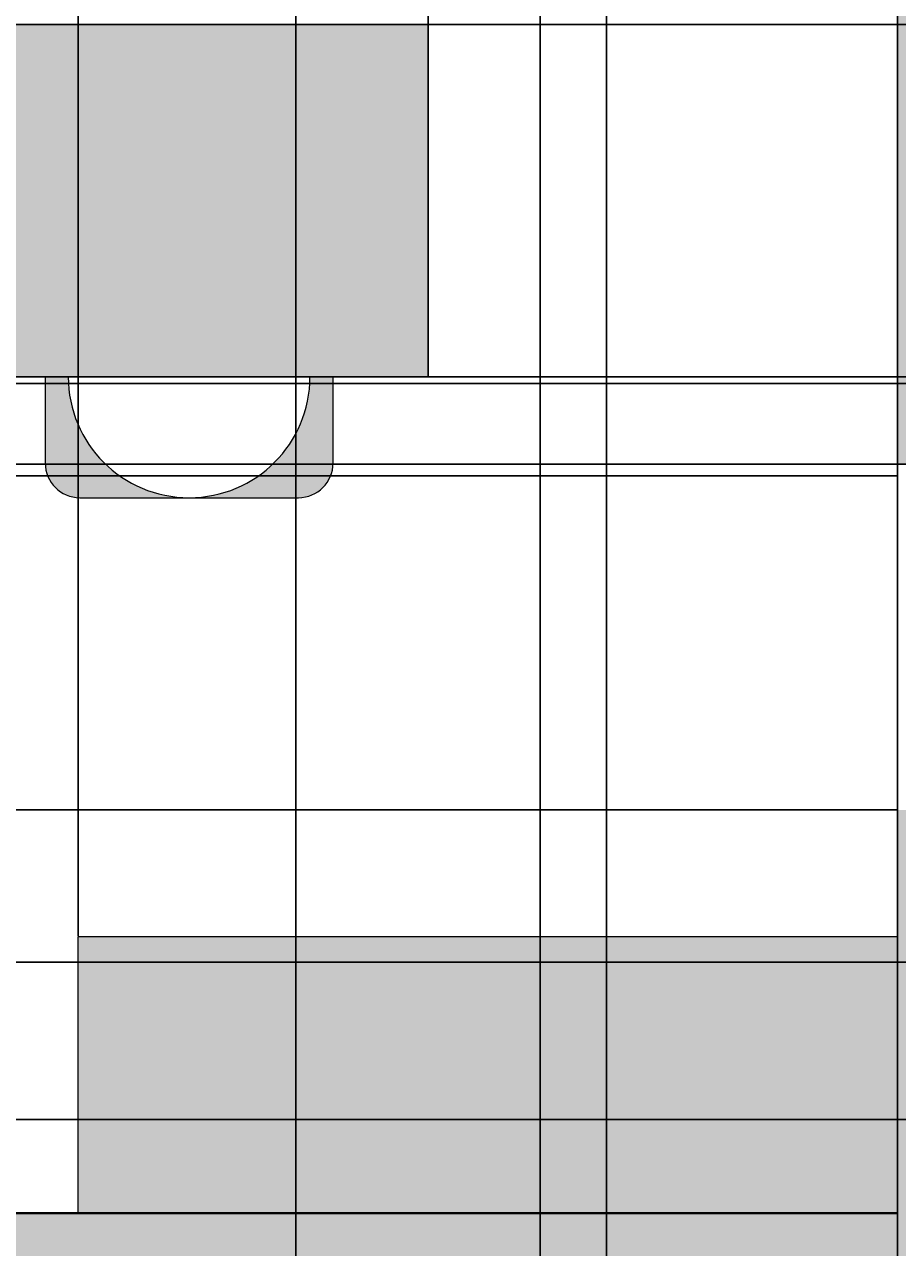
# Model space of a CAD drawing. Units: inches. Extents: x 818 to 1898, y 976 to 2364.
# Tile 83 of 96: x 1515 to 1591, y 1873 to 1979. Entities that reach past the tile are written whole.
import ezdxf

# ---------------------------------------------------------------- set-up
doc = ezdxf.new("R2010")
doc.units = ezdxf.units.IN
doc.header["$LTSCALE"] = 5
doc.header["$MEASUREMENT"] = 0
for name, color, linetype, lineweight in [('A-ANNO-DIMS', 2, 'Continuous', 18), ('A-FLOR-CASE', 8, 'Continuous', 18), ('A-FURN', 8, 'Continuous', 18), ('A-FURN-PATT', 8, 'Continuous', 9), ('A-WALL', 7, 'Continuous', 40)]:
    doc.layers.add(name, color=color, linetype=linetype, lineweight=lineweight)
doc.layers.add('A-WALL-PATT', color=251, linetype='Continuous', lineweight=13, true_color=0x636466)
doc.styles.get("Standard").update_dxf_attribs({"font": 'arial.ttf'})
doc.dimstyles.get("Standard").update_dxf_attribs({"dimtxt": 0.18, "dimasz": 0.18, "dimexe": 0.18, "dimexo": 0.0625, "dimgap": 0.09, "dimtad": 0, "dimtih": 1, "dimtoh": 1, "dimdec": 4, "dimzin": 0, "dimdsep": 46, "dimtxsty": 'Standard', "dimcen": 0.09, "dimadec": 0, "dimazin": 0, "dimtfac": 1, "dimtdec": 4, "dimtofl": 0, "dimtmove": 0, "dimatfit": 3, "dimfxl": 1, "dimtolj": 1, "dimtzin": 0, "dimarcsym": 0})

# ---------------------------------------------------------------- blocks, each defined once
blk = doc.blocks.new('*D74')
at = {"layer": 'A-ANNO-DIMS', "color": 0, "lineweight": -2, "ltscale": 5, "transparency": 16777216}
for p, q in [((1590.66, 1940.08), (818.03, 1940.08)), ((818.21, 1939.9), (818.21, 1925.76)), ((818.21, 1911.26), (818.21, 1925.4)), ((1590.66, 1911.08), (818.03, 1911.08))]:
    blk.add_line(p, q, dxfattribs=at)
at = {"layer": 'A-ANNO-DIMS', "color": 0, "ltscale": 5, "transparency": 16777216}
for points in [[(818.18, 1939.9), (818.24, 1939.9), (818.21, 1940.08)], [(818.18, 1911.26), (818.24, 1911.26), (818.21, 1911.08)]]:
    blk.add_solid(points, dxfattribs=at)
at = {"layer": 'Defpoints', "color": 0, "ltscale": 5, "transparency": 16777216}
for p in [(818.21, 1940.08), (1590.73, 1940.08), (1590.73, 1911.08)]:
    blk.add_point(p, dxfattribs=at)
at = {"layer": 'A-ANNO-DIMS', "color": 0, "ltscale": 5, "transparency": 16777216, "insert": (818.21, 1925.58), "char_height": 0.18, "attachment_point": 5}
blk.add_mtext('\\A1;29', dxfattribs=at)
blk = doc.blocks.new('*D85')
at = {"layer": 'A-ANNO-DIMS', "color": 0, "lineweight": -2, "ltscale": 5, "transparency": 16777216}
for p, q in [((1258.79, 2053.08), (1897.92, 2053.08)), ((1897.74, 2052.9), (1897.74, 1876.76)), ((1897.74, 1700.26), (1897.74, 1876.4)), ((1258.79, 1700.08), (1897.92, 1700.08))]:
    blk.add_line(p, q, dxfattribs=at)
at = {"layer": 'A-ANNO-DIMS', "color": 0, "ltscale": 5, "transparency": 16777216}
for points in [[(1897.71, 2052.9), (1897.77, 2052.9), (1897.74, 2053.08)], [(1897.71, 1700.26), (1897.77, 1700.26), (1897.74, 1700.08)]]:
    blk.add_solid(points, dxfattribs=at)
at = {"layer": 'Defpoints', "color": 0, "ltscale": 5, "transparency": 16777216}
for p in [(1258.73, 2053.08), (1897.74, 2053.08), (1258.73, 1700.08)]:
    blk.add_point(p, dxfattribs=at)
at = {"layer": 'A-ANNO-DIMS', "color": 0, "ltscale": 5, "transparency": 16777216, "insert": (1897.74, 1876.58), "char_height": 0.18, "attachment_point": 5}
blk.add_mtext('\\A1;353', dxfattribs=at)
blk = doc.blocks.new('*D101')
at = {"layer": 'A-ANNO-DIMS', "color": 0, "lineweight": -2, "ltscale": 5, "transparency": 16777216}
for p, q in [((1507.3, 1071.12), (1507.3, 2363.87)), ((1507.48, 2363.69), (1536, 2363.69)), ((1565.3, 2363.69), (1536.78, 2363.69)), ((1565.48, 1071.12), (1565.48, 2363.87))]:
    blk.add_line(p, q, dxfattribs=at)
at = {"layer": 'A-ANNO-DIMS', "color": 0, "ltscale": 5, "transparency": 16777216}
for points in [[(1507.48, 2363.72), (1507.48, 2363.66), (1507.3, 2363.69)], [(1565.3, 2363.72), (1565.3, 2363.66), (1565.48, 2363.69)]]:
    blk.add_solid(points, dxfattribs=at)
at = {"layer": 'Defpoints', "color": 0, "ltscale": 5, "transparency": 16777216}
for p in [(1565.48, 2363.69), (1507.3, 1071.06), (1565.48, 1071.06)]:
    blk.add_point(p, dxfattribs=at)
at = {"layer": 'A-ANNO-DIMS', "color": 0, "ltscale": 5, "transparency": 16777216, "insert": (1536.39, 2363.69), "char_height": 0.18, "attachment_point": 5}
blk.add_mtext('\\A1;58.19', dxfattribs=at)
blk = doc.blocks.new('*D102')
at = {"layer": 'A-ANNO-DIMS', "color": 0, "lineweight": -2, "ltscale": 5, "transparency": 16777216}
for p, q in [((1565.48, 1071.12), (1565.48, 2363.87)), ((1565.66, 2363.69), (1595.63, 2363.69)), ((1626.39, 2363.69), (1596.42, 2363.69)), ((1626.57, 1071.12), (1626.57, 2363.87))]:
    blk.add_line(p, q, dxfattribs=at)
at = {"layer": 'A-ANNO-DIMS', "color": 0, "ltscale": 5, "transparency": 16777216}
for points in [[(1565.66, 2363.72), (1565.66, 2363.66), (1565.48, 2363.69)], [(1626.39, 2363.72), (1626.39, 2363.66), (1626.57, 2363.69)]]:
    blk.add_solid(points, dxfattribs=at)
at = {"layer": 'Defpoints', "color": 0, "ltscale": 5, "transparency": 16777216}
for p in [(1626.57, 2363.69), (1565.48, 1071.06), (1626.57, 1071.06)]:
    blk.add_point(p, dxfattribs=at)
at = {"layer": 'A-ANNO-DIMS', "color": 0, "ltscale": 5, "transparency": 16777216, "insert": (1596.03, 2363.69), "char_height": 0.18, "attachment_point": 5}
blk.add_mtext('\\A1;61.09', dxfattribs=at)
blk = doc.blocks.new('*D121')
at = {"layer": 'A-ANNO-DIMS', "color": 0, "lineweight": -2, "ltscale": 5, "transparency": 16777216}
for p, q in [((1766.29, 1884.2), (818.03, 1884.2)), ((818.21, 1884.02), (818.21, 1841.14)), ((818.21, 1797.9), (818.21, 1840.78)), ((1766.29, 1797.72), (818.03, 1797.72))]:
    blk.add_line(p, q, dxfattribs=at)
at = {"layer": 'A-ANNO-DIMS', "color": 0, "ltscale": 5, "transparency": 16777216}
for points in [[(818.18, 1884.02), (818.24, 1884.02), (818.21, 1884.2)], [(818.18, 1797.9), (818.24, 1797.9), (818.21, 1797.72)]]:
    blk.add_solid(points, dxfattribs=at)
at = {"layer": 'Defpoints', "color": 0, "ltscale": 5, "transparency": 16777216}
for p in [(818.21, 1884.2), (1766.35, 1884.2), (1766.35, 1797.72)]:
    blk.add_point(p, dxfattribs=at)
at = {"layer": 'A-ANNO-DIMS', "color": 0, "ltscale": 5, "transparency": 16777216, "insert": (818.21, 1840.96), "char_height": 0.18, "attachment_point": 5}
blk.add_mtext('\\A1;86.49', dxfattribs=at)
blk = doc.blocks.new('*D161')
at = {"layer": 'A-ANNO-DIMS', "color": 0, "lineweight": -2, "ltscale": 5, "transparency": 16777216}
for p, q in [((1429.23, 1876.14), (1429.23, 2363.87)), ((1429.41, 2363.69), (1509.59, 2363.69)), ((1590.55, 2363.69), (1510.36, 2363.69)), ((1590.73, 1876.14), (1590.73, 2363.87))]:
    blk.add_line(p, q, dxfattribs=at)
at = {"layer": 'A-ANNO-DIMS', "color": 0, "ltscale": 5, "transparency": 16777216}
for points in [[(1429.41, 2363.72), (1429.41, 2363.66), (1429.23, 2363.69)], [(1590.55, 2363.72), (1590.55, 2363.66), (1590.73, 2363.69)]]:
    blk.add_solid(points, dxfattribs=at)
at = {"layer": 'Defpoints', "color": 0, "ltscale": 5, "transparency": 16777216}
for p in [(1590.73, 2363.69), (1429.23, 1876.08), (1590.73, 1876.08)]:
    blk.add_point(p, dxfattribs=at)
at = {"layer": 'A-ANNO-DIMS', "color": 0, "ltscale": 5, "transparency": 16777216, "insert": (1509.98, 2363.69), "char_height": 0.18, "attachment_point": 5}
blk.add_mtext('\\A1;161.5', dxfattribs=at)
blk = doc.blocks.new('*D175')
at = {"layer": 'A-ANNO-DIMS', "color": 0, "lineweight": -2, "ltscale": 5, "transparency": 16777216}
for p, q in [((1559.73, 1647.64), (1559.73, 2363.87)), ((1559.91, 2363.69), (1614.45, 2363.69)), ((1669.55, 2363.69), (1615.01, 2363.69)), ((1669.73, 1647.64), (1669.73, 2363.87))]:
    blk.add_line(p, q, dxfattribs=at)
at = {"layer": 'A-ANNO-DIMS', "color": 0, "ltscale": 5, "transparency": 16777216}
for points in [[(1559.91, 2363.72), (1559.91, 2363.66), (1559.73, 2363.69)], [(1669.55, 2363.72), (1669.55, 2363.66), (1669.73, 2363.69)]]:
    blk.add_solid(points, dxfattribs=at)
at = {"layer": 'Defpoints', "color": 0, "ltscale": 5, "transparency": 16777216}
for p in [(1669.73, 2363.69), (1559.73, 1647.58), (1669.73, 1647.58)]:
    blk.add_point(p, dxfattribs=at)
at = {"layer": 'A-ANNO-DIMS', "color": 0, "ltscale": 5, "transparency": 16777216, "insert": (1614.73, 2363.69), "char_height": 0.18, "attachment_point": 5}
blk.add_mtext('\\A1;110', dxfattribs=at)
blk = doc.blocks.new('*D206')
at = {"layer": 'A-ANNO-DIMS', "color": 0, "lineweight": -2, "ltscale": 5, "transparency": 16777216}
for p, q in [((1590.66, 1911.08), (818.03, 1911.08)), ((818.21, 1910.9), (818.21, 1893.76)), ((818.21, 1876.26), (818.21, 1893.4)), ((1590.66, 1876.08), (818.03, 1876.08))]:
    blk.add_line(p, q, dxfattribs=at)
at = {"layer": 'A-ANNO-DIMS', "color": 0, "ltscale": 5, "transparency": 16777216}
for points in [[(818.18, 1910.9), (818.24, 1910.9), (818.21, 1911.08)], [(818.18, 1876.26), (818.24, 1876.26), (818.21, 1876.08)]]:
    blk.add_solid(points, dxfattribs=at)
at = {"layer": 'Defpoints', "color": 0, "ltscale": 5, "transparency": 16777216}
for p in [(818.21, 1911.08), (1590.73, 1911.08), (1590.73, 1876.08)]:
    blk.add_point(p, dxfattribs=at)
at = {"layer": 'A-ANNO-DIMS', "color": 0, "ltscale": 5, "transparency": 16777216, "insert": (818.21, 1893.58), "char_height": 0.18, "attachment_point": 5}
blk.add_mtext('\\A1;35', dxfattribs=at)
blk = doc.blocks.new('*D211')
at = {"layer": 'A-ANNO-DIMS', "color": 0, "lineweight": -2, "ltscale": 5, "transparency": 16777216}
for p, q in [((1599.66265, 1948.078237), (818.025912, 1948.078237)), ((818.205912, 1947.898237), (818.205912, 1944.758237)), ((818.205912, 1941.258237), (818.205912, 1944.398237)), ((1599.66265, 1941.078237), (818.025912, 1941.078237))]:
    blk.add_line(p, q, dxfattribs=at)
at = {"layer": 'A-ANNO-DIMS', "color": 0, "ltscale": 5, "transparency": 16777216}
for points in [[(818.175912, 1947.898237), (818.235912, 1947.898237), (818.205912, 1948.078237)], [(818.175912, 1941.258237), (818.235912, 1941.258237), (818.205912, 1941.078237)]]:
    blk.add_solid(points, dxfattribs=at)
at = {"layer": 'Defpoints', "color": 0, "ltscale": 5, "transparency": 16777216}
for p in [(818.205912, 1948.078237), (1599.72515, 1948.078237), (1599.72515, 1941.078237)]:
    blk.add_point(p, dxfattribs=at)
at = {"layer": 'A-ANNO-DIMS', "color": 0, "ltscale": 5, "transparency": 16777216, "insert": (818.205912, 1944.578237), "char_height": 0.18, "attachment_point": 5}
blk.add_mtext('\\A1;7', dxfattribs=at)
blk = doc.blocks.new('*D215')
at = {"layer": 'A-ANNO-DIMS', "color": 0, "lineweight": -2, "ltscale": 5, "transparency": 16777216}
for p, q in [((1590.66, 1876.08), (818.03, 1876.08)), ((818.21, 1875.9), (818.21, 1781.76)), ((818.21, 1687.26), (818.21, 1781.4)), ((1511.66, 1687.08), (818.03, 1687.08))]:
    blk.add_line(p, q, dxfattribs=at)
at = {"layer": 'A-ANNO-DIMS', "color": 0, "ltscale": 5, "transparency": 16777216}
for points in [[(818.18, 1875.9), (818.24, 1875.9), (818.21, 1876.08)], [(818.18, 1687.26), (818.24, 1687.26), (818.21, 1687.08)]]:
    blk.add_solid(points, dxfattribs=at)
at = {"layer": 'Defpoints', "color": 0, "ltscale": 5, "transparency": 16777216}
for p in [(818.21, 1876.08), (1590.73, 1876.08), (1511.73, 1687.08)]:
    blk.add_point(p, dxfattribs=at)
at = {"layer": 'A-ANNO-DIMS', "color": 0, "ltscale": 5, "transparency": 16777216, "insert": (818.21, 1781.58), "char_height": 0.18, "attachment_point": 5}
blk.add_mtext('\\A1;189', dxfattribs=at)
blk = doc.blocks.new('*D238')
at = {"layer": 'A-ANNO-DIMS', "color": 0, "lineweight": -2, "ltscale": 5, "transparency": 16777216}
for p, q in [((1483.55, 1948.72), (1483.55, 2363.87)), ((1483.73, 2363.69), (1516.38, 2363.69)), ((1549.83, 2363.69), (1517.17, 2363.69)), ((1550.01, 1948.72), (1550.01, 2363.87))]:
    blk.add_line(p, q, dxfattribs=at)
at = {"layer": 'A-ANNO-DIMS', "color": 0, "ltscale": 5, "transparency": 16777216}
for points in [[(1483.73, 2363.72), (1483.73, 2363.66), (1483.55, 2363.69)], [(1549.83, 2363.72), (1549.83, 2363.66), (1550.01, 2363.69)]]:
    blk.add_solid(points, dxfattribs=at)
at = {"layer": 'Defpoints', "color": 0, "ltscale": 5, "transparency": 16777216}
for p in [(1550.01, 2363.69), (1483.55, 1948.66), (1550.01, 1948.66)]:
    blk.add_point(p, dxfattribs=at)
at = {"layer": 'A-ANNO-DIMS', "color": 0, "ltscale": 5, "transparency": 16777216, "insert": (1516.78, 2363.69), "char_height": 0.18, "attachment_point": 5}
blk.add_mtext('\\A1;66.47', dxfattribs=at)
blk = doc.blocks.new('*D239')
at = {"layer": 'A-ANNO-DIMS', "color": 0, "lineweight": -2, "ltscale": 5, "transparency": 16777216}
for p, q in [((1483.61, 1979.24), (1897.92, 1979.24)), ((1897.74, 1979.06), (1897.74, 1964.13)), ((1897.74, 1948.84), (1897.74, 1963.77)), ((1483.61, 1948.66), (1897.92, 1948.66))]:
    blk.add_line(p, q, dxfattribs=at)
at = {"layer": 'A-ANNO-DIMS', "color": 0, "ltscale": 5, "transparency": 16777216}
for points in [[(1897.71, 1979.06), (1897.77, 1979.06), (1897.74, 1979.24)], [(1897.71, 1948.84), (1897.77, 1948.84), (1897.74, 1948.66)]]:
    blk.add_solid(points, dxfattribs=at)
at = {"layer": 'Defpoints', "color": 0, "ltscale": 5, "transparency": 16777216}
for p in [(1483.55, 1979.24), (1897.74, 1979.24), (1483.55, 1948.66)]:
    blk.add_point(p, dxfattribs=at)
at = {"layer": 'A-ANNO-DIMS', "color": 0, "ltscale": 5, "transparency": 16777216, "insert": (1897.74, 1963.95), "char_height": 0.18, "attachment_point": 5}
blk.add_mtext('\\A1;30.584', dxfattribs=at)
blk = doc.blocks.new('*D243')
at = {"layer": 'A-ANNO-DIMS', "color": 0, "lineweight": -2, "ltscale": 5, "transparency": 16777216}
for p, q in [((1451.77, 2020.02), (1451.77, 975.66)), ((1590.73, 2020.02), (1590.73, 975.66)), ((1451.95, 975.84), (1520.79, 975.84)), ((1590.55, 975.84), (1521.7, 975.84))]:
    blk.add_line(p, q, dxfattribs=at)
at = {"layer": 'A-ANNO-DIMS', "color": 0, "ltscale": 5, "transparency": 16777216}
for points in [[(1451.95, 975.87), (1451.95, 975.81), (1451.77, 975.84)], [(1590.55, 975.87), (1590.55, 975.81), (1590.73, 975.84)]]:
    blk.add_solid(points, dxfattribs=at)
at = {"layer": 'Defpoints', "color": 0, "ltscale": 5, "transparency": 16777216}
for p in [(1451.77, 2020.08), (1590.73, 2020.08), (1590.73, 975.84)]:
    blk.add_point(p, dxfattribs=at)
at = {"layer": 'A-ANNO-DIMS', "color": 0, "ltscale": 5, "transparency": 16777216, "insert": (1521.25, 975.84), "char_height": 0.18, "attachment_point": 5}
blk.add_mtext('\\A1;138.96', dxfattribs=at)
blk = doc.blocks.new('*D244')
at = {"layer": 'A-ANNO-DIMS', "color": 0, "lineweight": -2, "ltscale": 5, "transparency": 16777216}
for p, q in [((1519.64, 1900.14), (1519.64, 2363.87)), ((1519.82, 2363.69), (1554.79, 2363.69)), ((1590.55, 2363.69), (1555.58, 2363.69)), ((1590.73, 1900.14), (1590.73, 2363.87))]:
    blk.add_line(p, q, dxfattribs=at)
at = {"layer": 'A-ANNO-DIMS', "color": 0, "ltscale": 5, "transparency": 16777216}
for points in [[(1519.82, 2363.72), (1519.82, 2363.66), (1519.64, 2363.69)], [(1590.55, 2363.72), (1590.55, 2363.66), (1590.73, 2363.69)]]:
    blk.add_solid(points, dxfattribs=at)
at = {"layer": 'Defpoints', "color": 0, "ltscale": 5, "transparency": 16777216}
for p in [(1590.73, 2363.69), (1519.64, 1900.08), (1590.73, 1900.08)]:
    blk.add_point(p, dxfattribs=at)
at = {"layer": 'A-ANNO-DIMS', "color": 0, "ltscale": 5, "transparency": 16777216, "insert": (1555.18, 2363.69), "char_height": 0.18, "attachment_point": 5}
blk.add_mtext('\\A1;71.08', dxfattribs=at)
blk = doc.blocks.new('*D253')
at = {"layer": 'A-ANNO-DIMS', "color": 0, "lineweight": -2, "ltscale": 5, "transparency": 16777216}
for p, q in [((1485.12, 2053.02), (1485.12, 975.66)), ((1538.52, 2053.02), (1538.52, 975.66)), ((1485.3, 975.84), (1511.42, 975.84)), ((1538.34, 975.84), (1512.21, 975.84))]:
    blk.add_line(p, q, dxfattribs=at)
at = {"layer": 'A-ANNO-DIMS', "color": 0, "ltscale": 5, "transparency": 16777216}
for points in [[(1485.3, 975.87), (1485.3, 975.81), (1485.12, 975.84)], [(1538.34, 975.87), (1538.34, 975.81), (1538.52, 975.84)]]:
    blk.add_solid(points, dxfattribs=at)
at = {"layer": 'Defpoints', "color": 0, "ltscale": 5, "transparency": 16777216}
for p in [(1485.12, 2053.08), (1538.52, 2053.08), (1538.52, 975.84)]:
    blk.add_point(p, dxfattribs=at)
at = {"layer": 'A-ANNO-DIMS', "color": 0, "ltscale": 5, "transparency": 16777216, "insert": (1511.82, 975.84), "char_height": 0.18, "attachment_point": 5}
blk.add_mtext('\\A1;53.39', dxfattribs=at)
blk = doc.blocks.new('*D275')
at = {"layer": 'A-ANNO-DIMS', "color": 0, "lineweight": -2, "ltscale": 5, "transparency": 16777216}
for p, q in [((1377.84, 1897.87), (1897.92, 1897.87)), ((1897.74, 1897.69), (1897.74, 1875.99)), ((1897.74, 1853.93), (1897.74, 1875.63)), ((1377.84, 1853.75), (1897.92, 1853.75))]:
    blk.add_line(p, q, dxfattribs=at)
at = {"layer": 'A-ANNO-DIMS', "color": 0, "ltscale": 5, "transparency": 16777216}
for points in [[(1897.71, 1897.69), (1897.77, 1897.69), (1897.74, 1897.87)], [(1897.71, 1853.93), (1897.77, 1853.93), (1897.74, 1853.75)]]:
    blk.add_solid(points, dxfattribs=at)
at = {"layer": 'Defpoints', "color": 0, "ltscale": 5, "transparency": 16777216}
for p in [(1377.78, 1897.87), (1897.74, 1897.87), (1377.78, 1853.75)]:
    blk.add_point(p, dxfattribs=at)
at = {"layer": 'A-ANNO-DIMS', "color": 0, "ltscale": 5, "transparency": 16777216, "insert": (1897.74, 1875.81), "char_height": 0.18, "attachment_point": 5}
blk.add_mtext('\\A1;44.12', dxfattribs=at)
blk = doc.blocks.new('*D281')
at = {"layer": 'A-ANNO-DIMS', "color": 0, "lineweight": -2, "ltscale": 5, "transparency": 16777216}
for p, q in [((1250.3, 1913.7), (1250.3, 2363.87)), ((1250.48, 2363.69), (1420.12, 2363.69)), ((1590.55, 2363.69), (1420.91, 2363.69)), ((1590.73, 2011.14), (1590.73, 2363.87))]:
    blk.add_line(p, q, dxfattribs=at)
at = {"layer": 'A-ANNO-DIMS', "color": 0, "ltscale": 5, "transparency": 16777216}
for points in [[(1250.48, 2363.72), (1250.48, 2363.66), (1250.3, 2363.69)], [(1590.55, 2363.72), (1590.55, 2363.66), (1590.73, 2363.69)]]:
    blk.add_solid(points, dxfattribs=at)
at = {"layer": 'Defpoints', "color": 0, "ltscale": 5, "transparency": 16777216}
for p in [(1590.73, 2363.69), (1590.73, 2011.08), (1250.3, 1913.64)]:
    blk.add_point(p, dxfattribs=at)
at = {"layer": 'A-ANNO-DIMS', "color": 0, "ltscale": 5, "transparency": 16777216, "insert": (1420.51, 2363.69), "char_height": 0.18, "attachment_point": 5}
blk.add_mtext('\\A1;340.4', dxfattribs=at)
blk = doc.blocks.new('*D282')
at = {"layer": 'A-ANNO-DIMS', "color": 0, "lineweight": -2, "ltscale": 5, "transparency": 16777216}
for p, q in [((1422.08, 2081.19), (1897.92, 2081.19)), ((1897.74, 2081.01), (1897.74, 1884.32)), ((1897.74, 1687.26), (1897.74, 1883.95)), ((1463.79, 1687.08), (1897.92, 1687.08))]:
    blk.add_line(p, q, dxfattribs=at)
at = {"layer": 'A-ANNO-DIMS', "color": 0, "ltscale": 5, "transparency": 16777216}
for points in [[(1897.71, 2081.01), (1897.77, 2081.01), (1897.74, 2081.19)], [(1897.71, 1687.26), (1897.77, 1687.26), (1897.74, 1687.08)]]:
    blk.add_solid(points, dxfattribs=at)
at = {"layer": 'Defpoints', "color": 0, "ltscale": 5, "transparency": 16777216}
for p in [(1422.02, 2081.19), (1897.74, 2081.19), (1463.73, 1687.08)]:
    blk.add_point(p, dxfattribs=at)
at = {"layer": 'A-ANNO-DIMS', "color": 0, "ltscale": 5, "transparency": 16777216, "insert": (1897.74, 1884.13), "char_height": 0.18, "attachment_point": 5}
blk.add_mtext('\\A1;394.1', dxfattribs=at)

msp = doc.modelspace()

# ---------------------------------------------------------------- hatches: boundary and pattern name
at = {"layer": 'A-FURN-PATT', "ltscale": 5}
h = msp.add_hatch(color=256, dxfattribs=at)
h.dxf.hatch_style = 1
h.paths.add_polyline_path([(1341.9997, 1981.5338), (1317.9034, 2001.8247), (1314.2595, 2001.8247), (1314.2595, 2004.893), (1310.1046, 2008.3917), (1303.9314, 2008.3917), (1303.9314, 1953.0408), (1308.1629, 1953.0408), (1314.2595, 1958.1746), (1314.2595, 1959.6079), (1315.9616, 1959.6079)])
h.paths.add_polyline_path([(1341.9997, 1981.5338), (1315.9616, 1959.6079), (1336.7936, 1959.6079), (1336.7936, 1953.0408), (1345.3966, 1953.0408), (1345.3966, 1959.6079), (1368.0379, 1959.6079)])
h.paths.add_polyline_path([(1402.518, 2008.3917), (1398.8475, 2008.3917), (1398.8475, 2001.8247), (1376.3134, 2001.8247), (1376.3134, 2008.3917), (1373.8948, 2008.3917), (1367.9307, 2003.3695), (1367.9307, 2001.8247), (1366.0961, 2001.8247), (1341.9997, 1981.5338), (1368.0379, 1959.6079), (1375.8366, 1953.0408), (1376.3134, 1953.0408), (1376.3134, 1959.6079), (1398.8475, 1959.6079), (1398.8475, 1953.0408), (1402.518, 1953.0408)])
h.paths.add_polyline_path([(1366.0961, 2001.8247), (1345.3966, 2001.8247), (1345.3966, 2008.3917), (1336.7936, 2008.3917), (1336.7936, 2001.8247), (1317.9034, 2001.8247), (1341.9997, 1981.5338)])
h.paths.add_polyline_path([(1336.7936, 1959.6079), (1315.9616, 1959.6079), (1314.2595, 1958.1746), (1314.2595, 1953.0408), (1336.7936, 1953.0408)], flags=17)
h.paths.add_polyline_path([(1367.9307, 1959.6079), (1345.3966, 1959.6079), (1345.3966, 1953.0408), (1367.9307, 1953.0408)], flags=17)
h.paths.add_polyline_path([(1398.8475, 1959.6079), (1376.3134, 1959.6079), (1376.3134, 1953.0408), (1398.8475, 1953.0408)], flags=17)
h.paths.add_polyline_path([(1368.0379, 1959.6079), (1367.9307, 1959.6079), (1367.9307, 1953.0408), (1375.8366, 1953.0408)], flags=17)
h.paths.add_polyline_path([(1314.2595, 1958.1746), (1308.1629, 1953.0408), (1314.2595, 1953.0408)], flags=17)
h.paths.add_polyline_path([(1315.9616, 1959.6079), (1314.2595, 1959.6079), (1314.2595, 1958.1746)], flags=16)
h.paths.add_polyline_path([(1314.2595, 2008.3917), (1310.1046, 2008.3917), (1314.2595, 2004.893)], flags=17)
h.paths.add_polyline_path([(1336.7936, 2008.3917), (1314.2595, 2008.3917), (1314.2595, 2004.893), (1317.9034, 2001.8247), (1336.7936, 2001.8247)], flags=17)
h.paths.add_polyline_path([(1314.2595, 2004.893), (1314.2595, 2001.8247), (1317.9034, 2001.8247)], flags=16)
h.paths.add_polyline_path([(1367.9307, 2008.3917), (1345.3966, 2008.3917), (1345.3966, 2001.8247), (1366.0961, 2001.8247), (1367.9307, 2003.3695)], flags=17)
h.paths.add_polyline_path([(1398.8475, 2008.3917), (1376.3134, 2008.3917), (1376.3134, 2001.8247), (1398.8475, 2001.8247)], flags=17)
h.paths.add_polyline_path([(1373.8948, 2008.3917), (1367.9307, 2008.3917), (1367.9307, 2003.3695)], flags=17)
h.paths.add_polyline_path([(1367.9307, 2003.3695), (1366.0961, 2001.8247), (1367.9307, 2001.8247)], flags=16)
h.paths.add_polyline_path([(1546.1595, 2044.0782), (1451.7698, 2044.0782), (1451.7698, 2020.0782), (1546.1595, 2020.0782)])
h.paths.add_polyline_path([(1492.0729, 2040.001, 0.431429), (1491.8238, 2040.251), (1491.3087, 2040.251, 0.41521699), (1491.0729, 2040.001)], flags=16)
h.paths.add_polyline_path([(1481.8346, 2039.6036), (1511.886, 2039.6036), (1511.886, 2024.9917), (1481.8346, 2024.9917)], flags=16)
h.paths.add_polyline_path([(1491.0729, 2039.4857), (1491.0729, 2039.501), (1492.0729, 2039.501, -0.41174844), (1491.8401, 2039.251), (1491.8229, 2039.251), (1491.8229, 2039.2509, 0.43259178), (1492.0729, 2039.501), (1491.0729, 2039.501, 0.43260402), (1491.3229, 2039.2509), (1491.3229, 2039.251), (1491.325, 2039.251, -0.41658228)], flags=0)
h.paths.add_polyline_path([(1485.3701, 2030.9622), (1485.3701, 2034.3556, -0.41421356), (1488.3701, 2037.3556), (1490.3421, 2037.3556, -0.07791932), (1491.0729, 2038.751), (1495.0729, 2038.751, -0.31486788), (1496.07, 2037.1201, -0.30166092), (1497.9049, 2034.3556), (1497.9049, 2030.9622, -0.41421356), (1494.9049, 2027.9622), (1488.3701, 2027.9622, -0.41421356)], flags=0)
h.paths.add_polyline_path([(1490.3229, 2035.751, 0.26556482), (1491.3229, 2036.751), (1491.3229, 2037.126), (1491.0729, 2037.126, -0.79141832), (1490.5434, 2037.251, -0.79141832), (1491.0729, 2037.376), (1491.3229, 2037.376), (1491.3229, 2037.751), (1492.0729, 2037.751), (1492.0729, 2037.376), (1492.3229, 2037.376, -0.79141832), (1492.8524, 2037.251, -0.79141832), (1492.3229, 2037.126), (1492.1491, 2037.126, -0.08662632), (1492.5376, 2036.0294, 0.10704809), (1493.0729, 2035.751), (1490.3229, 2035.751)], flags=0)
h.paths.add_polyline_path([(1491.9774, 2037.251, -1), (1491.4184, 2037.251, -1)], flags=0)
h.paths.add_polyline_path([(1500.0743, 2028.6045), (1500.0743, 2029.4074), (1510.8414, 2029.4074), (1510.8414, 2028.6045)], flags=0)
h.paths.add_polyline_path([(1500.0743, 2030.5314), (1500.0743, 2031.3342), (1510.8414, 2031.3342), (1510.8414, 2030.5314)], flags=0)
h.paths.add_polyline_path([(1500.0743, 2032.94), (1500.0743, 2033.7428), (1510.8414, 2033.7428), (1510.8414, 2032.94)], flags=0)
h.paths.add_polyline_path([(1500.0743, 2035.7499), (1500.0743, 2036.5528), (1510.8414, 2036.5528), (1510.8414, 2035.7499)], flags=0)
h.paths.add_polyline_path([(1590.7251, 2044.0782), (1576.1595, 2044.0782), (1576.1595, 2020.0782), (1590.7251, 2020.0782)])
h.paths.add_polyline_path([(1668.4429, 2044.0782), (1599.7251, 2044.0782), (1599.7251, 2020.0782), (1668.4429, 2020.0782)])
h.paths.add_polyline_path([(1621.2588, 2040.001, 0.431429), (1621.0097, 2040.251), (1620.4946, 2040.251, 0.41521699), (1620.2588, 2040.001)], flags=16)
h.paths.add_polyline_path([(1611.0205, 2024.9917), (1611.0205, 2039.6036), (1641.0719, 2039.6036), (1641.0719, 2024.9917)], flags=16)
h.paths.add_polyline_path([(1620.2588, 2039.4857), (1620.2588, 2039.501), (1621.2588, 2039.501, -0.41174844), (1621.026, 2039.251), (1621.0088, 2039.251), (1621.0088, 2039.2509, 0.43259178), (1621.2588, 2039.501), (1620.2588, 2039.501, 0.43260402), (1620.5088, 2039.2509), (1620.5088, 2039.251), (1620.5109, 2039.251, -0.41658228)], flags=0)
h.paths.add_polyline_path([(1614.556, 2030.9622), (1614.556, 2034.3556, -0.41421356), (1617.556, 2037.3556), (1619.528, 2037.3556, -0.07791932), (1620.2588, 2038.751), (1624.2588, 2038.751, -0.31486788), (1625.2559, 2037.1201, -0.30166092), (1627.0908, 2034.3556), (1627.0908, 2030.9622, -0.41421356), (1624.0908, 2027.9622), (1617.556, 2027.9622, -0.41421356)], flags=0)
h.paths.add_polyline_path([(1619.5088, 2035.751, 0.26556482), (1620.5088, 2036.751), (1620.5088, 2037.126), (1620.2588, 2037.126, -0.79141832), (1619.7293, 2037.251, -0.79141832), (1620.2588, 2037.376), (1620.5088, 2037.376), (1620.5088, 2037.751), (1621.2588, 2037.751), (1621.2588, 2037.376), (1621.5088, 2037.376, -0.79141832), (1622.0383, 2037.251, -0.79141832), (1621.5088, 2037.126), (1621.335, 2037.126, -0.08662632), (1621.7235, 2036.0294, 0.10704809), (1622.2588, 2035.751), (1619.5088, 2035.751)], flags=0)
h.paths.add_polyline_path([(1620.6043, 2037.251, -1), (1621.1633, 2037.251, -1)], flags=0)
h.paths.add_polyline_path([(1629.2602, 2028.6045), (1629.2602, 2029.4074), (1640.0273, 2029.4074), (1640.0273, 2028.6045)], flags=0)
h.paths.add_polyline_path([(1629.2602, 2030.5314), (1629.2602, 2031.3342), (1640.0273, 2031.3342), (1640.0273, 2030.5314)], flags=0)
h.paths.add_polyline_path([(1629.2602, 2032.94), (1629.2602, 2033.7428), (1640.0273, 2033.7428), (1640.0273, 2032.94)], flags=0)
h.paths.add_polyline_path([(1629.2602, 2035.7499), (1629.2602, 2036.5528), (1640.0273, 2036.5528), (1640.0273, 2035.7499)], flags=0)
h.paths.add_polyline_path([(1705.7252, 2044.0782), (1698.4429, 2044.0782), (1698.4429, 2020.0782), (1705.7252, 2020.0782)])
h.paths.add_polyline_path([(1705.7252, 1972.0782), (1599.7251, 1972.0782), (1599.7251, 1948.0782), (1705.7252, 1948.0782)])
h.paths.add_polyline_path([(1550.0109, 1979.2444), (1483.5451, 1979.2444), (1483.5451, 1948.6602), (1550.0109, 1948.6602)])
h.paths.add_polyline_path([(1490.2586, 1948.6602), (1488.2586, 1948.6602), (1488.2586, 1941.1742, 0.41421356), (1491.2586, 1938.1742), (1500.7446, 1938.1742, -0.41421356)])
h.paths.add_polyline_path([(1513.2306, 1941.1742), (1513.2306, 1948.6602), (1511.2306, 1948.6602, -0.41421356), (1500.7446, 1938.1742), (1510.2306, 1938.1742, 0.41421356)])
h.paths.add_polyline_path([(1518.778, 1948.6602), (1516.778, 1948.6602), (1516.778, 1941.1742, 0.41421356), (1519.778, 1938.1742), (1529.264, 1938.1742, -0.41421356)])
h.paths.add_polyline_path([(1541.75, 1941.1742), (1541.75, 1948.6602), (1539.75, 1948.6602, -0.41421356), (1529.264, 1938.1742), (1538.75, 1938.1742, 0.41421356)])
h.paths.add_polyline_path([(1590.7251, 1900.0782), (1519.6413, 1900.0782), (1519.6413, 1876.0782), (1590.7251, 1876.0782)])
at = {"layer": 'A-WALL-PATT', "ltscale": 5}
h = msp.add_hatch(color=256, dxfattribs=at)
h.dxf.hatch_style = 1
h.paths.add_polyline_path([(1267.7252, 1928.9218), (1258.7251, 1928.9218), (1258.7251, 1913.6401), (1250.3029, 1913.6401), (1250.3029, 1878.3919), (1258.7251, 1878.3919), (1258.7251, 1862.9652), (1267.7252, 1862.9652)])
h.paths.add_polyline_path([(1267.7252, 1814.9652), (1258.7251, 1814.9652), (1258.7251, 1755.3321), (1267.7252, 1755.3321)])
h.paths.add_polyline_path([(1463.7251, 1696.0782), (1267.7252, 1696.0782), (1267.7252, 1707.3321), (1258.7251, 1707.3321), (1258.7251, 1700.0782), (1251.9333, 1700.0782), (1251.9333, 1687.0782), (1463.7251, 1687.0782)])
h.paths.add_polyline_path([(1714.7252, 1717.3178), (1705.7252, 1717.3178), (1705.7252, 1696.0782), (1599.7251, 1696.0782), (1599.7251, 1790.0782), (1705.7252, 1790.0782), (1705.7252, 1785.6125), (1714.7252, 1785.6125), (1714.7252, 1827.2125), (1705.7252, 1827.2125), (1705.7252, 1802.0782), (1599.7251, 1802.0782), (1599.7251, 1867.0782), (1705.7252, 1867.0782), (1705.7252, 1857.2125), (1714.7252, 1857.2125), (1714.7252, 1930.0316), (1741.8409, 1930.0316), (1741.8409, 1935.0316), (1714.7252, 1935.0316), (1714.7252, 1957.0338), (1741.8409, 1957.0338), (1741.8409, 1962.0338), (1714.7252, 1962.0338), (1705.7252, 1962.0338), (1705.7252, 1948.0782), (1599.7251, 1948.0782), (1599.7251, 1981.0782), (1590.7251, 1981.0782), (1590.7251, 1941.0782), (1620.7252, 1941.0782), (1705.7252, 1941.0782), (1705.7252, 1876.0782), (1599.7251, 1876.0782), (1599.7251, 1911.0782), (1590.7251, 1911.0782), (1590.7251, 1876.0782), (1429.2251, 1876.0782), (1429.2251, 1867.0782), (1511.7251, 1867.0782), (1528.593, 1867.0782), (1595.7252, 1867.0782), (1595.7252, 1773.0782), (1520.7252, 1773.0782), (1520.7252, 1837.5823), (1532.593, 1837.5823), (1532.593, 1867.0782), (1528.593, 1867.0782), (1528.593, 1841.5823), (1511.7251, 1841.5823), (1511.7251, 1744.9714), (1520.7252, 1744.9714), (1520.7252, 1761.0782), (1595.7252, 1761.0782), (1595.7252, 1696.0782), (1520.7252, 1696.0782), (1520.7252, 1716.0454), (1511.7251, 1716.0454), (1511.7251, 1696.0782), (1511.7251, 1687.0782), (1714.7252, 1687.0782)])
h.paths.add_polyline_path([(1714.7252, 2053.0782), (1714.7252, 2081.1881), (1709.7252, 2081.1881), (1709.7252, 2053.0782), (1681.6446, 2053.0782), (1681.6446, 2081.1881), (1676.6446, 2081.1881), (1676.6446, 2053.0782), (1538.5155, 2053.0782), (1538.5155, 2044.0782), (1590.7251, 2044.0782), (1590.7251, 2011.0782), (1599.7251, 2011.0782), (1599.7251, 2044.0782), (1705.7252, 2044.0782), (1705.7252, 2014.5114), (1714.7252, 2014.5114)])
h.paths.add_polyline_path([(1485.1216, 2053.0782), (1422.02, 2053.0782), (1422.02, 2081.1881), (1413.02, 2081.1881), (1413.02, 2053.0782), (1399.6356, 2053.0782), (1399.6356, 2081.1881), (1390.6356, 2081.1881), (1390.6356, 2053.0782), (1388.0315, 2053.0782), (1388.0315, 2044.0782), (1416.2743, 2044.0782), (1485.1216, 2044.0782)])
h.paths.add_polyline_path([(1330.305, 2053.0782), (1258.7251, 2053.0782), (1258.7251, 2019.2871), (1267.7252, 2019.2871), (1267.7252, 2044.0782), (1330.305, 2044.0782)])
h.paths.add_polyline_path([(1258.7251, 2053.0782), (1214.6577, 2053.0782), (1214.6577, 2044.0782), (1258.7251, 2044.0782)])
h.paths.add_polyline_path([(1214.6577, 2053.0782), (1180.349, 2053.0782), (1180.349, 2044.0782), (1214.6577, 2044.0782)])
h.paths.add_polyline_path([(1714.7252, 1639.5782), (1741.8409, 1639.5782), (1741.8409, 1643.5782), (1714.7252, 1643.5782), (1714.7252, 1649.9029), (1705.7252, 1649.9029), (1705.7252, 1600.0782), (1477.7252, 1600.0782), (1477.7252, 1591.0782), (1520.7252, 1591.0782), (1616.7252, 1591.0782), (1616.7252, 1416.6857), (1622.7252, 1416.6857), (1622.7252, 1463.0782), (1624.7252, 1463.0782), (1624.7252, 1467.0782), (1622.7252, 1467.0782), (1622.7252, 1591.0782), (1705.7252, 1591.0782), (1705.7252, 1545.0782), (1714.7252, 1545.0782), (1741.8409, 1545.0782), (1741.8409, 1549.0782), (1714.7252, 1549.0782), (1714.7252, 1593.9175), (1737.8409, 1593.9175), (1737.8409, 1597.9175), (1714.7252, 1597.9175)])
h.paths.add_polyline_path([(1674.9024, 2060.7419), (1714.7045, 2060.7419), (1714.7045, 2073.1061), (1674.9024, 2073.1061)], flags=25)
h.paths.add_polyline_path([(1394.5468, 2061.6618), (1422.2344, 2061.6618), (1422.2344, 2074.0261), (1394.5468, 2074.0261)], flags=24)

# ---------------------------------------------------------------- linework, layer by layer
at = {"layer": 'A-FLOR-CASE'}
for p, q in [((1519.6413, 1900.0782), (1590.7251, 1900.0782)), ((1519.6413, 1876.0782), (1519.6413, 1900.0782))]:
    msp.add_line(p, q, dxfattribs=at)
msp.add_lwpolyline([(1483.5451, 1979.2444), (1550.0109, 1979.2444), (1550.0109, 1948.6602), (1483.5451, 1948.6602)], close=True, dxfattribs=at)
at = {"layer": 'A-FURN'}
for p, q in [((1518.778, 1948.6602), (1516.778, 1948.6602)), ((1516.778, 1948.6602), (1516.778, 1941.1742)), ((1541.75, 1941.1742), (1541.75, 1948.6602)), ((1519.778, 1938.1742), (1529.264, 1938.1742)), ((1529.264, 1938.1742), (1538.75, 1938.1742))]:
    msp.add_line(p, q, dxfattribs=at)
for centre, radius, start, end in [((1529.264, 1948.6602), 10.486, 180, 0), ((1519.778, 1941.1742), 3, 180, 270), ((1538.75, 1941.1742), 3, 270, 0)]:
    msp.add_arc(centre, radius, start, end, dxfattribs=at)
at = {"layer": 'A-WALL'}
msp.add_line((1429.2251, 1876.0782), (1590.7251, 1876.0782), dxfattribs=at)

# ---------------------------------------------------------------- dimensions: what is measured, and where the dimension line sits
at = {"layer": 'A-ANNO-DIMS', "ltscale": 5}
for base, p1, p2, override, picture, middle in [((1590.7251, 2363.6929), (1250.3029, 1913.6401), (1590.7251, 2011.0782), {"dimdec": 1, "dimlfac": 1, "dimrnd": 0, "dimzin": 0, "dimdsep": 46, "dimlunit": 2}, '*D281', (1420.514, 2363.6929)), ((1590.7251, 2363.6929), (1429.2251, 1876.0782), (1590.7251, 1876.0782), {"dimdec": 1, "dimlfac": 1, "dimrnd": 0, "dimzin": 0, "dimdsep": 46, "dimlunit": 2}, '*D161', (1509.9751, 2363.6929)), ((1550.0109, 2363.6929), (1483.5451, 1948.6602), (1550.0109, 1948.6602), {"dimdec": 2, "dimlfac": 1, "dimrnd": 0, "dimzin": 0, "dimdsep": 46, "dimlunit": 2}, '*D238', (1516.778, 2363.6929)), ((1565.4835, 2363.6929), (1507.2982, 1071.0552), (1565.4835, 1071.0552), {"dimdec": 2, "dimlfac": 1, "dimrnd": 0, "dimzin": 0, "dimdsep": 46, "dimlunit": 2}, '*D101', (1536.3908, 2363.6929)), ((1590.7251, 2363.6929), (1519.6413, 1900.0782), (1590.7251, 1900.0782), {"dimdec": 2, "dimlfac": 1, "dimrnd": 0, "dimzin": 0, "dimdsep": 46, "dimlunit": 2}, '*D244', (1555.1832, 2363.6929)), ((1669.7251, 2363.6929), (1559.7251, 1647.5782), (1669.7251, 1647.5782), {"dimdec": 0, "dimlfac": 1, "dimrnd": 0, "dimzin": 0, "dimdsep": 46, "dimlunit": 2}, '*D175', (1614.7251, 2363.6929)), ((1626.5748, 2363.6929), (1565.4835, 1071.0552), (1626.5748, 1071.0552), {"dimdec": 2, "dimlfac": 1, "dimrnd": 0, "dimzin": 0, "dimdsep": 46, "dimlunit": 2}, '*D102', (1596.0291, 2363.6929)), ((1538.5155, 975.8433), (1485.1216, 2053.0782), (1538.5155, 2053.0782), {"dimdec": 2, "dimlfac": 1, "dimrnd": 0, "dimzin": 0, "dimdsep": 46, "dimlunit": 2}, '*D253', (1511.8185, 975.8433)), ((1590.7251, 975.8433), (1451.7698, 2020.0782), (1590.7251, 2020.0782), {"dimdec": 2, "dimlfac": 1, "dimrnd": 0, "dimzin": 0, "dimdsep": 46, "dimlunit": 2}, '*D243', (1521.2475, 975.8433))]:
    dim = msp.add_linear_dim(base=base, p1=p1, p2=p2, dimstyle='Standard', override=override, dxfattribs=at)
    dim.commit()
    dim.dimension.update_dxf_attribs({"geometry": picture, "text_midpoint": middle})
for base, p1, p2, override, picture, middle in [((1897.736, 2081.1881), (1463.7251, 1687.0782), (1422.02, 2081.1881), {"dimdec": 1, "dimlfac": 1, "dimrnd": 0, "dimzin": 0, "dimdsep": 46, "dimlunit": 2}, '*D282', (1897.736, 1884.1332)), ((1897.736, 2053.0782), (1258.7251, 1700.0782), (1258.7251, 2053.0782), {"dimdec": 0, "dimlfac": 1, "dimrnd": 0, "dimzin": 0, "dimdsep": 46, "dimlunit": 2}, '*D85', (1897.736, 1876.5782)), ((1897.736, 1979.2444), (1483.5451, 1948.6602), (1483.5451, 1979.2444), {"dimdec": 3, "dimlfac": 1, "dimrnd": 0, "dimzin": 0, "dimdsep": 46, "dimlunit": 2}, '*D239', (1897.736, 1963.9523)), ((818.2059, 1948.0782), (1599.7251, 1941.0782), (1599.7251, 1948.0782), {"dimdec": 0, "dimlfac": 1, "dimrnd": 0, "dimzin": 0, "dimdsep": 46, "dimlunit": 2}, '*D211', (818.2059, 1944.5782)), ((818.2059, 1940.0782), (1590.7251, 1911.0782), (1590.7251, 1940.0782), {"dimdec": 0, "dimlfac": 1, "dimrnd": 0, "dimzin": 0, "dimdsep": 46, "dimlunit": 2}, '*D74', (818.2059, 1925.5782)), ((818.2059, 1911.0782), (1590.7251, 1876.0782), (1590.7251, 1911.0782), {"dimdec": 0, "dimlfac": 1, "dimrnd": 0, "dimzin": 0, "dimdsep": 46, "dimlunit": 2}, '*D206', (818.2059, 1893.5782)), ((1897.736, 1897.8663), (1377.7791, 1853.7496), (1377.7791, 1897.8663), {"dimdec": 2, "dimlfac": 1, "dimrnd": 0, "dimzin": 0, "dimdsep": 46, "dimlunit": 2}, '*D275', (1897.736, 1875.808)), ((818.2059, 1884.2031), (1766.3524, 1797.7165), (1766.3524, 1884.2031), {"dimdec": 2, "dimlfac": 1, "dimrnd": 0, "dimzin": 0, "dimdsep": 46, "dimlunit": 2}, '*D121', (818.2059, 1840.9598)), ((818.2059, 1876.0782), (1511.7251, 1687.0782), (1590.7251, 1876.0782), {"dimdec": 0, "dimlfac": 1, "dimrnd": 0, "dimzin": 0, "dimdsep": 46, "dimlunit": 2}, '*D215', (818.2059, 1781.5782))]:
    dim = msp.add_linear_dim(base=base, p1=p1, p2=p2, angle=90, dimstyle='Standard', override=override, dxfattribs=at)
    dim.commit()
    dim.dimension.update_dxf_attribs({"geometry": picture, "text_midpoint": middle})

doc.saveas('drawing.dxf')
